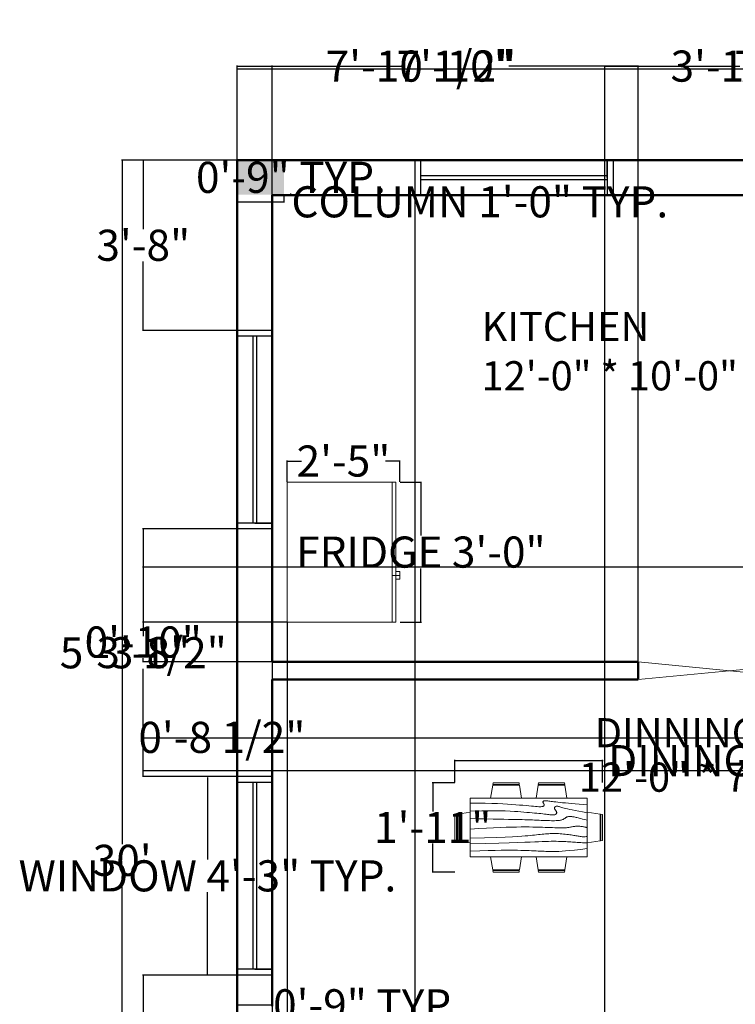
# Model space of a CAD drawing. Units: inches. Extents: x 9717 to 10218, y 17835 to 18358.
# Tile 2 of 4: x 9717 to 9901, y 18104 to 18358. Entities that reach past the tile are written whole.
import ezdxf

# ---------------------------------------------------------------- set-up
doc = ezdxf.new("R2010")
doc.units = ezdxf.units.IN
for name, color, linetype, lineweight in [('A-AREA-IDEN', 3, 'Continuous', 25), ('A-EQPM', 2, 'Continuous', 18), ('ARCHES', 5, 'Continuous', 18), ('COLUMN', 7, 'Continuous', 35), ('DIMENSIONS', 3, 'Continuous', 18), ('FURNITURES', 2, 'Continuous', 18), ('WALLS', 7, 'Continuous', 50), ('WINDOWS', 4, 'Continuous', 25)]:
    doc.layers.add(name, color=color, linetype=linetype, lineweight=lineweight)
doc.styles.get("Standard").update_dxf_attribs({"font": 'arial.ttf'})
doc.dimstyles.get("Standard").update_dxf_attribs({"dimtxt": 8, "dimasz": 0.18, "dimexe": 0.18, "dimexo": 0.0625, "dimgap": 0.09, "dimtad": 0, "dimtih": 1, "dimtoh": 1, "dimzin": 0, "dimdsep": 46, "dimlunit": 3, "dimtxsty": 'Standard', "dimcen": 0.09, "dimadec": 0, "dimazin": 0, "dimtfac": 1, "dimtofl": 0, "dimtmove": 0, "dimatfit": 3, "dimfxl": 1, "dimtolj": 1, "dimtzin": 0, "dimarcsym": 0})

# ---------------------------------------------------------------- blocks, each defined once
blk = doc.blocks.new('Dining Set - 36 x 72 in.')
for p, q in [((-22.2343, 26.00059), (-23.4847, 17.99762)), ((-22.2304, 26), (-5.7608, 26)), ((-22, 27.5), (-22.1562, 26.50042)), ((-5.8416, 26.5), (-22.1534, 26.5)), ((-22, 27.5), (-6, 27.5)), ((-5.8437, 26.49966), (-6, 27.5)), ((-4.5152, 17.99762), (-5.7655, 25.99926)), ((5.7657, 26.00059), (4.5153, 17.99762)), ((5.7696, 26), (22.2392, 26)), ((6, 27.5), (5.8438, 26.50042)), ((22.1584, 26.5), (5.8466, 26.5)), ((6, 27.5), (22, 27.5)), ((22.1563, 26.49966), (22, 27.5)), ((23.4848, 17.99762), (22.2345, 25.99926)), ((36, 18), (-36, 18)), ((-36, 18), (-36, -18)), ((36, -18), (36, 18)), ((-45.5, 8), (-44.5004, 8.15617)), ((-45.5, 8), (-45.5, -8)), ((-44.5, -8.15843), (-44.5, 8.15338)), ((-44.0006, 8.23428), (-35.9976, 9.48474)), ((-44, 8.23041), (-44, -8.23915)), ((44.0006, 8.23428), (35.9976, 9.48474)), ((44, 8.23041), (44, -8.23915)), ((44.5, -8.15843), (44.5, 8.15338)), ((45.5, 8), (44.5005, 8.15617)), ((45.5, 8), (45.5, -8)), ((-44.4997, -8.15631), (-45.5, -8)), ((-35.9976, -9.48476), (-43.9993, -8.2345)), ((35.9976, -9.48476), (43.9993, -8.2345)), ((44.4997, -8.15631), (45.5, -8)), ((-36, -18), (36, -18)), ((-22.2343, -26.0006), (-23.4847, -17.99762)), ((-4.5152, -17.99762), (-5.7655, -25.99928)), ((5.7657, -26.0006), (4.5153, -17.99762)), ((23.4848, -17.99762), (22.2345, -25.99928)), ((-22.2304, -26), (-5.7608, -26)), ((-22, -27.5), (-22.1562, -26.50044)), ((-5.8416, -26.5), (-22.1534, -26.5)), ((-22, -27.5), (-6, -27.5)), ((-5.8437, -26.49967), (-6, -27.5)), ((5.7696, -26), (22.2392, -26)), ((6, -27.5), (5.8438, -26.50044)), ((22.1584, -26.5), (5.8466, -26.5)), ((6, -27.5), (22, -27.5)), ((22.1563, -26.49967), (22, -27.5))]:
    blk.add_line(p, q)
for points in [[(-36, 15), (-31.1772, 14.97754), (-26.8079, 14.91406), (-22.8538, 14.81543), (-19.276, 14.6875), (-16.0362, 14.53613), (-13.0957, 14.36718), (-10.4159, 14.18652), (-7.9583, 14), (-5.6904, 13.81315), (-3.6035, 13.63021), (-1.6954, 13.45508), (0.0365, 13.29166), (1.5945, 13.14388), (2.9811, 13.01562), (4.1988, 12.9108), (5.25, 12.83333), (6.1393, 12.78613), (6.8802, 12.76823), (7.4883, 12.77767), (7.9792, 12.8125), (8.3685, 12.87077), (8.6719, 12.95052), (8.9049, 13.0498), (9.0833, 13.16666), (9.2205, 13.29899), (9.3216, 13.44401), (9.3895, 13.59879), (9.4271, 13.76041), (9.4373, 13.92594), (9.4232, 14.09245), (9.3875, 14.257), (9.3333, 14.41666), (9.2638, 14.56917), (9.1836, 14.71484), (9.0975, 14.85465), (9.0104, 14.98958), (8.9272, 15.1206), (8.8529, 15.2487), (8.7922, 15.37483), (8.75, 15.5), (8.7305, 15.62467), (8.7344, 15.74739), (8.7617, 15.86621), (8.8125, 15.97916), (8.8867, 16.08431), (8.9844, 16.17968), (9.1055, 16.26334), (9.25, 16.33333), (9.4189, 16.38802), (9.6172, 16.42708), (9.8506, 16.45052), (10.125, 16.45833), (10.4463, 16.45052), (10.8203, 16.42708), (11.2529, 16.38802), (11.75, 16.33333), (12.3184, 16.26318), (12.9694, 16.17838), (13.7151, 16.07991), (14.5677, 15.96875), (15.5395, 15.84586), (16.6426, 15.71224), (17.8893, 15.56884), (19.2917, 15.41666), (20.859, 15.25667), (22.5879, 15.08984), (24.4721, 14.91715), (26.5052, 14.73958), (28.6809, 14.5581), (30.9929, 14.3737), (33.4347, 14.18733), (36, 14)], [(-36, 10), (-28.9766, 10.14274), (-23.1725, 10.20442), (-18.4241, 10.19775), (-14.5677, 10.13541), (-11.4399, 10.03011), (-8.877, 9.89453), (-6.7154, 9.74137), (-4.7917, 9.58333), (-2.9698, 9.43082), (-1.2246, 9.28515), (0.4415, 9.14534), (2.026, 9.01041), (3.5266, 8.87939), (4.9408, 8.7513), (6.266, 8.62516), (7.5, 8.5), (8.6411, 8.37549), (9.6914, 8.2539), (10.6538, 8.13818), (11.5312, 8.03125), (12.3267, 7.93603), (13.043, 7.85547), (13.6831, 7.79248), (14.25, 7.75), (14.7471, 7.7303), (15.1797, 7.73307), (15.5537, 7.75732), (15.875, 7.80208), (16.1494, 7.86637), (16.3828, 7.94922), (16.5811, 8.04964), (16.75, 8.16666), (16.8944, 8.29915), (17.0143, 8.44531), (17.1089, 8.60319), (17.1771, 8.77083), (17.218, 8.94629), (17.2305, 9.1276), (17.2137, 9.31282), (17.1667, 9.5), (17.0895, 9.6875), (16.987, 9.875), (16.8649, 10.0625), (16.7292, 10.25), (16.5856, 10.4375), (16.4401, 10.625), (16.2985, 10.8125), (16.1667, 11), (16.05, 11.18733), (15.9518, 11.3737), (15.8752, 11.5581), (15.8229, 11.73958), (15.798, 11.91715), (15.8034, 12.08984), (15.842, 12.25667), (15.9167, 12.41666), (16.0295, 12.56836), (16.1784, 12.70833), (16.3605, 12.83268), (16.5729, 12.9375), (16.8127, 13.01888), (17.0768, 13.07291), (17.3625, 13.0957), (17.6667, 13.08333), (17.9894, 13.03312), (18.3418, 12.94726), (18.7382, 12.82918), (19.1927, 12.68229), (19.7195, 12.51001), (20.3327, 12.31575), (21.0465, 12.10294), (21.875, 11.875), (22.8357, 11.63354), (23.959, 11.37304), (25.2786, 11.08618), (26.8282, 10.76562), (28.6414, 10.40405), (30.752, 9.99414), (33.1936, 9.52856), (36, 9)], [(-36, 5.5), (-30.7157, 5.3348), (-26.069, 5.20963), (-21.9946, 5.11767), (-18.4271, 5.05208), (-15.3009, 5.00602), (-12.5508, 4.97265), (-10.1112, 4.94515), (-7.9167, 4.91666), (-5.909, 4.88167), (-4.0586, 4.83984), (-2.3429, 4.79215), (-0.7396, 4.73958), (0.7739, 4.6831), (2.22, 4.6237), (3.6213, 4.56233), (5, 4.5), (6.373, 4.43782), (7.7344, 4.3776), (9.0723, 4.32129), (10.375, 4.27083), (11.6309, 4.22819), (12.8281, 4.19531), (13.9551, 4.17415), (15, 4.16666), (15.954, 4.17448), (16.819, 4.19791), (17.6001, 4.23698), (18.3021, 4.29166), (18.9299, 4.36198), (19.4883, 4.44791), (19.9823, 4.54948), (20.4167, 4.66666), (20.7969, 4.79899), (21.1302, 4.94401), (21.4245, 5.09879), (21.6875, 5.26041), (21.9271, 5.42594), (22.1511, 5.59245), (22.3672, 5.757), (22.5834, 5.91666), (22.8065, 6.06868), (23.0404, 6.21093), (23.2879, 6.34147), (23.5521, 6.45833), (23.8358, 6.55957), (24.142, 6.64323), (24.4735, 6.70735), (24.8334, 6.75), (25.2235, 6.76969), (25.642, 6.76692), (26.0858, 6.74267), (26.5521, 6.69791), (27.0379, 6.63362), (27.5404, 6.55078), (28.0565, 6.45036), (28.5834, 6.33333), (29.1242, 6.19987), (29.7071, 6.04687), (30.3661, 5.87044), (31.1354, 5.66666), (32.0493, 5.43164), (33.142, 5.16146), (34.4475, 4.85221), (36, 4.5)], [(-36, -1), (-30.7915, -0.6591), (-26.0195, -0.38216), (-21.6519, -0.16284), (-17.6563, 0.00521), (-14.0005, 0.12833), (-10.6523, 0.21289), (-7.5796, 0.26522), (-4.75, 0.29166), (-2.134, 0.29793), (0.2878, 0.28711), (2.5317, 0.26163), (4.6146, 0.22396), (6.5529, 0.17651), (8.3633, 0.12174), (10.0623, 0.06209), (11.6667, 0), (13.1899, -0.06201), (14.6341, -0.1211), (15.9982, -0.17432), (17.2813, -0.21875), (18.4823, -0.25147), (19.6003, -0.26953), (20.6343, -0.27002), (21.5834, -0.25), (22.4481, -0.20768), (23.2357, -0.14584), (23.9549, -0.06836), (24.6146, 0.02083), (25.2235, 0.11784), (25.7904, 0.21875), (26.3241, 0.31966), (26.8334, 0.41666), (27.3265, 0.50618), (27.8099, 0.58593), (28.2894, 0.65397), (28.7709, 0.70833), (29.2601, 0.74707), (29.763, 0.76823), (30.2855, 0.76985), (30.8334, 0.75), (31.4088, 0.70784), (31.9994, 0.64713), (32.589, 0.57275), (33.1615, 0.48958), (33.7008, 0.4025), (34.1908, 0.3164), (34.6153, 0.23616), (34.9584, 0.16666), (35.2099, 0.11165), (35.3848, 0.07031), (35.504, 0.04069), (35.5886, 0.02083), (35.6594, 0.00879), (35.7377, 0.0026), (35.8442, 0.00032), (36, 0)], [(-36, -6.5), (-27.1843, -6.31267), (-20.084, -6.1263), (-14.469, -5.9419), (-10.1094, -5.76042), (-6.7752, -5.58285), (-4.2363, -5.41016), (-2.2629, -5.24333), (-0.625, -5.08334), (0.8708, -4.93099), (2.2715, -4.78646), (3.5872, -4.64974), (4.8281, -4.52084), (6.0046, -4.39974), (7.127, -4.28646), (8.2053, -4.18099), (9.25, -4.08334), (10.2705, -3.99382), (11.2734, -3.91407), (12.2647, -3.84603), (13.25, -3.79167), (14.2354, -3.75293), (15.2266, -3.73177), (16.2295, -3.73015), (17.25, -3.75), (18.2912, -3.79248), (19.3451, -3.85547), (20.4009, -3.93604), (21.4479, -4.03125), (22.4754, -4.13819), (23.4727, -4.25391), (24.4289, -4.37549), (25.3334, -4.5), (26.1785, -4.62492), (26.9694, -4.74935), (27.7145, -4.87281), (28.4219, -4.99479), (29.1, -5.11483), (29.7572, -5.23242), (30.4016, -5.34709), (31.0417, -5.45834), (31.6837, -5.56437), (32.3262, -5.65821), (32.9658, -5.73153), (33.599, -5.77604), (34.2224, -5.78345), (34.8327, -5.74545), (35.4264, -5.65373), (36, -5.5)], [(-36, -10), (-26.4022, -9.81299), (-18.4675, -9.62891), (-11.9839, -9.45069), (-6.7396, -9.28125), (-2.5226, -9.12354), (0.8789, -8.98047), (3.6769, -8.85498), (6.0833, -8.75), (8.2767, -8.66765), (10.3021, -8.60677), (12.1712, -8.56543), (13.8958, -8.54167), (15.4876, -8.53353), (16.9583, -8.53907), (18.3197, -8.55632), (19.5834, -8.58334), (20.7616, -8.61841), (21.8685, -8.66081), (22.9188, -8.71004), (23.9271, -8.76563), (24.9081, -8.82707), (25.8763, -8.89388), (26.8465, -8.96558), (27.8334, -9.04167), (28.8474, -9.12118), (29.8828, -9.20117), (30.93, -9.27824), (31.9792, -9.34896), (33.0205, -9.40991), (34.0443, -9.45768), (35.0407, -9.48885), (36, -9.5)], [(-36, -14.5), (-30.0881, -14.33513), (-25.0332, -14.21224), (-20.7312, -14.12647), (-17.0781, -14.07292), (-13.97, -14.04671), (-11.3027, -14.04297), (-8.9724, -14.05681), (-6.875, -14.08334), (-4.9224, -14.11833), (-3.0905, -14.16016), (-1.3709, -14.20785), (0.2448, -14.26042), (1.7647, -14.3169), (3.1973, -14.3763), (4.5507, -14.43767), (5.8333, -14.5), (7.0554, -14.5621), (8.235, -14.62175), (9.3922, -14.67652), (10.5469, -14.72396), (11.7192, -14.76164), (12.929, -14.78711), (14.1965, -14.79794), (15.5417, -14.79167), (16.9933, -14.76424), (18.6152, -14.70508), (20.4804, -14.60197), (22.6615, -14.44271), (25.2312, -14.21509), (28.2624, -13.9069), (31.8277, -13.50594), (36, -13)]]:
    blk.add_lwpolyline(points)
blk = doc.blocks.new('Refrigerator-2 door - 36 in top')
for p, q in [((0, -26.999999), (36, -26.999999)), ((12, -26.999999), (12, -28.999999)), ((11, -27.999999), (11, -28.999999)), ((11, -28.999999), (13, -28.999999)), ((13, -28.999999), (13, -27.999999))]:
    blk.add_line(p, q)
blk.add_lwpolyline([(0, -27.999999), (0, 0), (36, 0), (36, -27.999999)], close=True)
blk = doc.blocks.new('*D8')
at = {"layer": 'Defpoints', "color": 0, "transparency": 16777216}
for p in [(10150.76, 18344.92), (9772.76, 18321.49), (10150.76, 18321.49)]:
    blk.add_point(p, dxfattribs=at)
at = {"layer": 'DIMENSIONS', "color": 0, "lineweight": -2, "transparency": 16777216}
for p, q in [((9772.76, 18321.55), (9772.76, 18345.1)), ((9772.94, 18344.92), (9940.16, 18344.92)), ((10150.58, 18344.92), (9983.36, 18344.92)), ((10150.76, 18321.55), (10150.76, 18345.1))]:
    blk.add_line(p, q, dxfattribs=at)
at = {"layer": 'DIMENSIONS', "color": 0, "transparency": 16777216}
for points in [[(9772.94, 18344.95), (9772.94, 18344.89), (9772.76, 18344.92)], [(10150.58, 18344.95), (10150.58, 18344.89), (10150.76, 18344.92)]]:
    blk.add_solid(points, dxfattribs=at)
at = {"layer": 'DIMENSIONS', "color": 0, "transparency": 16777216, "insert": (9961.76, 18344.92), "char_height": 8, "attachment_point": 5}
blk.add_mtext('\\A1;31\'-6.00"', dxfattribs=at)
blk = doc.blocks.new('*D9')
at = {"layer": 'Defpoints', "color": 0, "transparency": 16777216}
for p in [(9772.76, 18321.49), (9743.19, 17961.49), (9772.76, 17961.49)]:
    blk.add_point(p, dxfattribs=at)
at = {"layer": 'DIMENSIONS', "color": 0, "lineweight": -2, "transparency": 16777216}
for p, q in [((9772.7, 18321.49), (9743.01, 18321.49)), ((9743.19, 18321.31), (9743.19, 18145.67)), ((9743.19, 17961.67), (9743.19, 18137.31)), ((9772.7, 17961.49), (9743.01, 17961.49))]:
    blk.add_line(p, q, dxfattribs=at)
at = {"layer": 'DIMENSIONS', "color": 0, "transparency": 16777216}
for points in [[(9743.16, 18321.31), (9743.22, 18321.31), (9743.19, 18321.49)], [(9743.16, 17961.67), (9743.22, 17961.67), (9743.19, 17961.49)]]:
    blk.add_solid(points, dxfattribs=at)
at = {"layer": 'DIMENSIONS', "color": 0, "transparency": 16777216, "insert": (9743.19, 18141.49), "char_height": 8, "attachment_point": 5}
blk.add_mtext("\\A1;30'", dxfattribs=at)
blk = doc.blocks.new('WIN-48IN')
for p, q in [((0.5, 9), (0, 9)), ((0, 9), (0, 0)), ((1, 9), (0.5, 9)), ((1.5, 9), (1, 9)), ((1.5, 9), (1.5, 0)), ((49.5, 4.5), (49.5, 9)), ((49.5, 9), (49.5, 0)), ((49.5, 9), (51, 9)), ((51, 9), (51, 0)), ((1.5, 5), (49.5, 5)), ((1.5, 4), (49.5, 4)), ((0, 0), (1.5, 0)), ((51, 0), (49.5, 0))]:
    blk.add_line(p, q)
blk = doc.blocks.new('COL-12X9IN')
h = blk.add_hatch(color=256)
h.dxf.hatch_style = 1
h.paths.add_polyline_path([(12, 0), (12, 9), (0, 9), (0, 0)])
blk = doc.blocks.new('*D14')
at = {"layer": 'Defpoints', "color": 0, "transparency": 16777216}
for p in [(9772.78, 18312.56), (9784.78, 18312.56), (9784.78, 18310.76)]:
    blk.add_point(p, dxfattribs=at)
at = {"layer": 'DIMENSIONS', "color": 0, "lineweight": -2, "transparency": 16777216}
for p, q in [((9772.78, 18312.5), (9772.78, 18310.58)), ((9772.96, 18310.76), (9784.6, 18310.76)), ((9784.78, 18312.5), (9784.78, 18310.58)), ((9784.78, 18310.76), (9784.96, 18310.76))]:
    blk.add_line(p, q, dxfattribs=at)
at = {"layer": 'DIMENSIONS', "color": 0, "transparency": 16777216}
for points in [[(9772.96, 18310.79), (9772.96, 18310.73), (9772.78, 18310.76)], [(9784.6, 18310.79), (9784.6, 18310.73), (9784.78, 18310.76)]]:
    blk.add_solid(points, dxfattribs=at)
at = {"layer": 'DIMENSIONS', "color": 0, "transparency": 16777216, "insert": (9835.15, 18310.76), "char_height": 8, "attachment_point": 5}
blk.add_mtext('\\A1;COLUMN 1\'-0" TYP.', dxfattribs=at)
blk = doc.blocks.new('*D15')
at = {"layer": 'Defpoints', "color": 0, "transparency": 16777216}
for p in [(9784.78, 18321.56), (9786.58, 18321.56), (9784.78, 18312.56)]:
    blk.add_point(p, dxfattribs=at)
at = {"layer": 'DIMENSIONS', "color": 0, "lineweight": -2, "transparency": 16777216}
for p, q in [((9784.84, 18321.56), (9786.76, 18321.56)), ((9786.58, 18321.38), (9786.58, 18321.23)), ((9786.58, 18312.74), (9786.58, 18312.88)), ((9784.84, 18312.56), (9786.76, 18312.56))]:
    blk.add_line(p, q, dxfattribs=at)
at = {"layer": 'DIMENSIONS', "color": 0, "transparency": 16777216}
for points in [[(9786.55, 18321.38), (9786.61, 18321.38), (9786.58, 18321.56)], [(9786.55, 18312.74), (9786.61, 18312.74), (9786.58, 18312.56)]]:
    blk.add_solid(points, dxfattribs=at)
at = {"layer": 'DIMENSIONS', "color": 0, "transparency": 16777216, "insert": (9786.58, 18317.06), "char_height": 8, "attachment_point": 5}
blk.add_mtext('\\A1;0\'-9" TYP.', dxfattribs=at)
blk = doc.blocks.new('*D16')
at = {"layer": 'Defpoints', "color": 0, "transparency": 16777216}
for p in [(9772.76, 18163.01), (9765.11, 18112.01), (9772.76, 18112.01)]:
    blk.add_point(p, dxfattribs=at)
at = {"layer": 'DIMENSIONS', "color": 0, "lineweight": -2, "transparency": 16777216}
for p, q in [((9772.7, 18163.01), (9764.93, 18163.01)), ((9765.11, 18162.83), (9765.11, 18141.74)), ((9765.11, 18112.19), (9765.11, 18133.28)), ((9772.7, 18112.01), (9764.93, 18112.01))]:
    blk.add_line(p, q, dxfattribs=at)
at = {"layer": 'DIMENSIONS', "color": 0, "transparency": 16777216}
for points in [[(9765.08, 18162.83), (9765.14, 18162.83), (9765.11, 18163.01)], [(9765.08, 18112.19), (9765.14, 18112.19), (9765.11, 18112.01)]]:
    blk.add_solid(points, dxfattribs=at)
at = {"layer": 'DIMENSIONS', "color": 0, "transparency": 16777216, "insert": (9765.11, 18137.51), "char_height": 8, "attachment_point": 5}
blk.add_mtext('\\A1;WINDOW 4\'-3" TYP.', dxfattribs=at)
blk = doc.blocks.new('*D17')
at = {"layer": 'Defpoints', "color": 0, "transparency": 16777216}
for p in [(9772.76, 18112.01), (9781.76, 18112.01), (9781.76, 18104.36)]:
    blk.add_point(p, dxfattribs=at)
at = {"layer": 'DIMENSIONS', "color": 0, "lineweight": -2, "transparency": 16777216}
for p, q in [((9772.76, 18111.95), (9772.76, 18104.18)), ((9781.76, 18111.95), (9781.76, 18104.18)), ((9772.94, 18104.36), (9781.58, 18104.36)), ((9781.76, 18104.36), (9781.94, 18104.36))]:
    blk.add_line(p, q, dxfattribs=at)
at = {"layer": 'DIMENSIONS', "color": 0, "transparency": 16777216}
for points in [[(9772.94, 18104.39), (9772.94, 18104.33), (9772.76, 18104.36)], [(9781.58, 18104.39), (9781.58, 18104.33), (9781.76, 18104.36)]]:
    blk.add_solid(points, dxfattribs=at)
at = {"layer": 'DIMENSIONS', "color": 0, "transparency": 16777216, "insert": (9806.41, 18104.36), "char_height": 8, "attachment_point": 5}
blk.add_mtext('\\A1;0\'-9" TYP.', dxfattribs=at)
blk = doc.blocks.new('*D28')
at = {"layer": 'Defpoints', "color": 0, "transparency": 16777216}
for p in [(9866.73, 18167.12), (9828.75, 18161.43), (9866.73, 18161.43)]:
    blk.add_point(p, dxfattribs=at)
at = {"layer": 'DIMENSIONS', "color": 0, "lineweight": -2, "transparency": 16777216}
for p, q in [((9828.75, 18161.49), (9828.75, 18167.3)), ((9828.93, 18167.12), (9866.55, 18167.12)), ((9866.73, 18161.49), (9866.73, 18167.3)), ((9866.73, 18167.12), (9866.91, 18167.12))]:
    blk.add_line(p, q, dxfattribs=at)
at = {"layer": 'DIMENSIONS', "color": 0, "transparency": 16777216}
for points in [[(9828.93, 18167.15), (9828.93, 18167.09), (9828.75, 18167.12)], [(9866.55, 18167.15), (9866.55, 18167.09), (9866.73, 18167.12)]]:
    blk.add_solid(points, dxfattribs=at)
at = {"layer": 'DIMENSIONS', "color": 0, "transparency": 16777216, "insert": (9910.97, 18167.12), "char_height": 8, "attachment_point": 5}
blk.add_mtext('\\A1;DINING SET 3\'-2"', dxfattribs=at)
blk = doc.blocks.new('*D29')
at = {"layer": 'Defpoints', "color": 0, "transparency": 16777216}
for p in [(9823.05, 18161.43), (9828.75, 18161.43), (9828.75, 18138.47)]:
    blk.add_point(p, dxfattribs=at)
at = {"layer": 'DIMENSIONS', "color": 0, "lineweight": -2, "transparency": 16777216}
for p, q in [((9828.69, 18161.43), (9822.87, 18161.43)), ((9823.05, 18161.25), (9823.05, 18154.05)), ((9823.05, 18138.65), (9823.05, 18145.84)), ((9828.69, 18138.47), (9822.87, 18138.47))]:
    blk.add_line(p, q, dxfattribs=at)
at = {"layer": 'DIMENSIONS', "color": 0, "transparency": 16777216}
for points in [[(9823.02, 18161.25), (9823.08, 18161.25), (9823.05, 18161.43)], [(9823.02, 18138.65), (9823.08, 18138.65), (9823.05, 18138.47)]]:
    blk.add_solid(points, dxfattribs=at)
at = {"layer": 'DIMENSIONS', "color": 0, "transparency": 16777216, "insert": (9823.05, 18149.95), "char_height": 8, "attachment_point": 5}
blk.add_mtext('\\A1;1\'-11"', dxfattribs=at)
blk = doc.blocks.new('*D30')
at = {"layer": 'Defpoints', "color": 0, "transparency": 16777216}
for p in [(9814.6, 18238.73), (9820, 18238.73), (9814.6, 18202.73)]:
    blk.add_point(p, dxfattribs=at)
at = {"layer": 'DIMENSIONS', "color": 0, "lineweight": -2, "transparency": 16777216}
for p, q in [((9814.66, 18238.73), (9820.18, 18238.73)), ((9820, 18238.55), (9820, 18224.96)), ((9820, 18202.91), (9820, 18216.51)), ((9814.66, 18202.73), (9820.18, 18202.73))]:
    blk.add_line(p, q, dxfattribs=at)
at = {"layer": 'DIMENSIONS', "color": 0, "transparency": 16777216}
for points in [[(9819.97, 18238.55), (9820.03, 18238.55), (9820, 18238.73)], [(9819.97, 18202.91), (9820.03, 18202.91), (9820, 18202.73)]]:
    blk.add_solid(points, dxfattribs=at)
at = {"layer": 'DIMENSIONS', "color": 0, "transparency": 16777216, "insert": (9820, 18220.73), "char_height": 8, "attachment_point": 5}
blk.add_mtext('\\A1;FRIDGE 3\'-0"', dxfattribs=at)
blk = doc.blocks.new('*D31')
at = {"layer": 'Defpoints', "color": 0, "transparency": 16777216}
for p in [(9785.6, 18244.13), (9785.6, 18238.73), (9814.6, 18238.73)]:
    blk.add_point(p, dxfattribs=at)
at = {"layer": 'DIMENSIONS', "color": 0, "lineweight": -2, "transparency": 16777216}
for p, q in [((9785.6, 18238.8), (9785.6, 18244.31)), ((9785.78, 18244.13), (9789.31, 18244.13)), ((9814.42, 18244.13), (9810.89, 18244.13)), ((9814.6, 18238.8), (9814.6, 18244.31))]:
    blk.add_line(p, q, dxfattribs=at)
at = {"layer": 'DIMENSIONS', "color": 0, "transparency": 16777216}
for points in [[(9785.78, 18244.16), (9785.78, 18244.1), (9785.6, 18244.13)], [(9814.42, 18244.16), (9814.42, 18244.1), (9814.6, 18244.13)]]:
    blk.add_solid(points, dxfattribs=at)
at = {"layer": 'DIMENSIONS', "color": 0, "transparency": 16777216, "insert": (9800.1, 18244.13), "char_height": 8, "attachment_point": 5}
blk.add_mtext('\\A1;2\'-5"', dxfattribs=at)
blk = doc.blocks.new('*D32')
at = {"layer": 'Defpoints', "color": 0, "transparency": 16777216}
for p in [(9867.28, 18345.64), (9867.28, 17970.49), (9772.76, 17961.49)]:
    blk.add_point(p, dxfattribs=at)
at = {"layer": 'DIMENSIONS', "color": 0, "lineweight": -2, "transparency": 16777216}
for p, q in [((9772.76, 17961.55), (9772.76, 18345.82)), ((9867.28, 17970.55), (9867.28, 18345.82)), ((9772.94, 18345.64), (9796.9, 18345.64)), ((9867.1, 18345.64), (9843.14, 18345.64))]:
    blk.add_line(p, q, dxfattribs=at)
at = {"layer": 'DIMENSIONS', "color": 0, "transparency": 16777216}
for points in [[(9772.94, 18345.67), (9772.94, 18345.61), (9772.76, 18345.64)], [(9867.1, 18345.67), (9867.1, 18345.61), (9867.28, 18345.64)]]:
    blk.add_solid(points, dxfattribs=at)
at = {"layer": 'DIMENSIONS', "color": 0, "transparency": 16777216, "insert": (9820.02, 18345.64), "char_height": 8, "attachment_point": 5}
blk.add_mtext('\\A1;7\'-10 1/2"', dxfattribs=at)
blk = doc.blocks.new('*D33')
at = {"layer": 'Defpoints', "color": 0, "transparency": 16777216}
for p in [(9958.06, 18345.64), (9867.28, 17970.49), (9958.06, 17970.49)]:
    blk.add_point(p, dxfattribs=at)
at = {"layer": 'DIMENSIONS', "color": 0, "lineweight": -2, "transparency": 16777216}
for p, q in [((9867.28, 17970.55), (9867.28, 18345.82)), ((9958.06, 17970.55), (9958.06, 18345.82)), ((9867.46, 18345.64), (9901.98, 18345.64)), ((9957.88, 18345.64), (9923.36, 18345.64))]:
    blk.add_line(p, q, dxfattribs=at)
at = {"layer": 'DIMENSIONS', "color": 0, "transparency": 16777216}
for points in [[(9867.46, 18345.67), (9867.46, 18345.61), (9867.28, 18345.64)], [(9957.88, 18345.67), (9957.88, 18345.61), (9958.06, 18345.64)]]:
    blk.add_solid(points, dxfattribs=at)
at = {"layer": 'DIMENSIONS', "color": 0, "transparency": 16777216, "insert": (9912.67, 18345.64), "char_height": 8, "attachment_point": 5}
blk.add_mtext('\\A1;7\'-7"', dxfattribs=at)
blk = doc.blocks.new('*D40')
at = {"layer": 'Defpoints', "color": 0, "transparency": 16777216}
for p in [(9781.76, 18312.49), (9818.43, 18312.49), (9818.43, 17847.34)]:
    blk.add_point(p, dxfattribs=at)
at = {"layer": 'DIMENSIONS', "color": 0, "lineweight": -2, "transparency": 16777216}
for p, q in [((9781.76, 18312.43), (9781.76, 17847.16)), ((9818.43, 18312.43), (9818.43, 17847.16)), ((9781.94, 17847.34), (9818.25, 17847.34)), ((9818.43, 17847.34), (9818.61, 17847.34))]:
    blk.add_line(p, q, dxfattribs=at)
at = {"layer": 'DIMENSIONS', "color": 0, "transparency": 16777216}
for points in [[(9781.94, 17847.37), (9781.94, 17847.31), (9781.76, 17847.34)], [(9818.25, 17847.37), (9818.25, 17847.31), (9818.43, 17847.34)]]:
    blk.add_solid(points, dxfattribs=at)
at = {"layer": 'DIMENSIONS', "color": 0, "transparency": 16777216, "insert": (9838.65, 17847.34), "char_height": 8, "attachment_point": 5}
blk.add_mtext('\\A1;3\'-0 1/2"', dxfattribs=at)
blk = doc.blocks.new('*D42')
at = {"layer": 'Defpoints', "color": 0, "transparency": 16777216}
for p in [(9772.76, 18321.49), (9748.61, 18277.7), (9772.76, 18277.7)]:
    blk.add_point(p, dxfattribs=at)
at = {"layer": 'DIMENSIONS', "color": 0, "lineweight": -2, "transparency": 16777216}
for p, q in [((9772.7, 18321.49), (9748.43, 18321.49)), ((9748.61, 18321.31), (9748.61, 18303.77)), ((9748.61, 18277.88), (9748.61, 18295.42)), ((9772.7, 18277.7), (9748.43, 18277.7))]:
    blk.add_line(p, q, dxfattribs=at)
at = {"layer": 'DIMENSIONS', "color": 0, "transparency": 16777216}
for points in [[(9748.58, 18321.31), (9748.64, 18321.31), (9748.61, 18321.49)], [(9748.58, 18277.88), (9748.64, 18277.88), (9748.61, 18277.7)]]:
    blk.add_solid(points, dxfattribs=at)
at = {"layer": 'DIMENSIONS', "color": 0, "transparency": 16777216, "insert": (9748.61, 18299.59), "char_height": 8, "attachment_point": 5}
blk.add_mtext('\\A1;3\'-8"', dxfattribs=at)
blk = doc.blocks.new('*D43')
at = {"layer": 'Defpoints', "color": 0, "transparency": 16777216}
for p in [(9748.61, 18226.7), (9772.76, 18226.7), (9772.76, 18163.01)]:
    blk.add_point(p, dxfattribs=at)
at = {"layer": 'DIMENSIONS', "color": 0, "lineweight": -2, "transparency": 16777216}
for p, q in [((9772.7, 18226.7), (9748.43, 18226.7)), ((9748.61, 18226.52), (9748.61, 18199.08)), ((9748.61, 18163.19), (9748.61, 18190.62)), ((9772.7, 18163.01), (9748.43, 18163.01))]:
    blk.add_line(p, q, dxfattribs=at)
at = {"layer": 'DIMENSIONS', "color": 0, "transparency": 16777216}
for points in [[(9748.58, 18226.52), (9748.64, 18226.52), (9748.61, 18226.7)], [(9748.58, 18163.19), (9748.64, 18163.19), (9748.61, 18163.01)]]:
    blk.add_solid(points, dxfattribs=at)
at = {"layer": 'DIMENSIONS', "color": 0, "transparency": 16777216, "insert": (9748.61, 18194.85), "char_height": 8, "attachment_point": 5}
blk.add_mtext('\\A1;5\'-3 1/2"', dxfattribs=at)
blk = doc.blocks.new('*D44')
at = {"layer": 'Defpoints', "color": 0, "transparency": 16777216}
for p in [(9748.61, 18112.01), (9772.76, 18112.01), (9772.76, 18056.11)]:
    blk.add_point(p, dxfattribs=at)
at = {"layer": 'DIMENSIONS', "color": 0, "lineweight": -2, "transparency": 16777216}
for p, q in [((9772.7, 18112.01), (9748.43, 18112.01)), ((9748.61, 18111.83), (9748.61, 18088.23)), ((9748.61, 18056.29), (9748.61, 18079.88)), ((9772.7, 18056.11), (9748.43, 18056.11))]:
    blk.add_line(p, q, dxfattribs=at)
at = {"layer": 'DIMENSIONS', "color": 0, "transparency": 16777216}
for points in [[(9748.58, 18111.83), (9748.64, 18111.83), (9748.61, 18112.01)], [(9748.58, 18056.29), (9748.64, 18056.29), (9748.61, 18056.11)]]:
    blk.add_solid(points, dxfattribs=at)
at = {"layer": 'DIMENSIONS', "color": 0, "transparency": 16777216, "insert": (9748.61, 18084.06), "char_height": 8, "attachment_point": 5}
blk.add_mtext('\\A1;4\'-8"', dxfattribs=at)
blk = doc.blocks.new('*D48')
at = {"layer": 'Defpoints', "color": 0, "transparency": 16777216}
for p in [(9875.9, 18345.64), (9781.76, 18192.49), (9875.9, 18192.49)]:
    blk.add_point(p, dxfattribs=at)
at = {"layer": 'DIMENSIONS', "color": 0, "lineweight": -2, "transparency": 16777216}
for p, q in [((9781.76, 18192.55), (9781.76, 18345.82)), ((9875.9, 18192.55), (9875.9, 18345.82)), ((9781.94, 18345.64), (9815.03, 18345.64)), ((9875.72, 18345.64), (9842.63, 18345.64))]:
    blk.add_line(p, q, dxfattribs=at)
at = {"layer": 'DIMENSIONS', "color": 0, "transparency": 16777216}
for points in [[(9781.94, 18345.67), (9781.94, 18345.61), (9781.76, 18345.64)], [(9875.72, 18345.67), (9875.72, 18345.61), (9875.9, 18345.64)]]:
    blk.add_solid(points, dxfattribs=at)
at = {"layer": 'DIMENSIONS', "color": 0, "transparency": 16777216, "insert": (9828.83, 18345.64), "char_height": 8, "attachment_point": 5}
blk.add_mtext('\\A1;7\'-10"', dxfattribs=at)
blk = doc.blocks.new('*D49')
at = {"layer": 'Defpoints', "color": 0, "transparency": 16777216}
for p in [(9922.68, 18345.64), (9875.9, 18192.49), (9922.68, 18192.49)]:
    blk.add_point(p, dxfattribs=at)
at = {"layer": 'DIMENSIONS', "color": 0, "lineweight": -2, "transparency": 16777216}
for p, q in [((9875.9, 18192.55), (9875.9, 18345.82)), ((9922.68, 18192.55), (9922.68, 18345.82)), ((9876.08, 18345.64), (9885.46, 18345.64)), ((9922.5, 18345.64), (9913.12, 18345.64))]:
    blk.add_line(p, q, dxfattribs=at)
at = {"layer": 'DIMENSIONS', "color": 0, "transparency": 16777216}
for points in [[(9876.08, 18345.67), (9876.08, 18345.61), (9875.9, 18345.64)], [(9922.5, 18345.67), (9922.5, 18345.61), (9922.68, 18345.64)]]:
    blk.add_solid(points, dxfattribs=at)
at = {"layer": 'DIMENSIONS', "color": 0, "transparency": 16777216, "insert": (9899.29, 18345.64), "char_height": 8, "attachment_point": 5}
blk.add_mtext('\\A1;3\'-11"', dxfattribs=at)
blk = doc.blocks.new('*D52')
at = {"layer": 'Defpoints', "color": 0, "transparency": 16777216}
for p in [(9748.61, 18216.87), (9993.26, 18216.87), (9993.26, 18172.92)]:
    blk.add_point(p, dxfattribs=at)
at = {"layer": 'DIMENSIONS', "color": 0, "lineweight": -2, "transparency": 16777216}
for p, q in [((9993.2, 18216.87), (9748.43, 18216.87)), ((9748.61, 18216.69), (9748.61, 18199.08)), ((9748.61, 18173.1), (9748.61, 18190.72)), ((9993.2, 18172.92), (9748.43, 18172.92))]:
    blk.add_line(p, q, dxfattribs=at)
at = {"layer": 'DIMENSIONS', "color": 0, "transparency": 16777216}
for points in [[(9748.58, 18216.69), (9748.64, 18216.69), (9748.61, 18216.87)], [(9748.58, 18173.1), (9748.64, 18173.1), (9748.61, 18172.92)]]:
    blk.add_solid(points, dxfattribs=at)
at = {"layer": 'DIMENSIONS', "color": 0, "transparency": 16777216, "insert": (9748.61, 18194.9), "char_height": 8, "attachment_point": 5}
blk.add_mtext('\\A1;3\'-8"', dxfattribs=at)
blk = doc.blocks.new('*D61')
at = {"layer": 'Defpoints', "color": 0, "transparency": 16777216}
for p in [(9748.61, 18172.92), (9993.26, 18172.92), (9993.26, 18164.49)]:
    blk.add_point(p, dxfattribs=at)
at = {"layer": 'DIMENSIONS', "color": 0, "lineweight": -2, "transparency": 16777216}
for p, q in [((9993.2, 18172.92), (9748.43, 18172.92)), ((9748.61, 18172.92), (9748.61, 18173.1)), ((9748.61, 18173.1), (9748.79, 18173.1)), ((9748.61, 18164.67), (9748.61, 18172.74)), ((9993.2, 18164.49), (9748.43, 18164.49))]:
    blk.add_line(p, q, dxfattribs=at)
at = {"layer": 'DIMENSIONS', "color": 0, "transparency": 16777216}
for points in [[(9748.58, 18172.74), (9748.64, 18172.74), (9748.61, 18172.92)], [(9748.58, 18164.67), (9748.64, 18164.67), (9748.61, 18164.49)]]:
    blk.add_solid(points, dxfattribs=at)
at = {"layer": 'DIMENSIONS', "color": 0, "transparency": 16777216, "insert": (9768.83, 18173.1), "char_height": 8, "attachment_point": 5}
blk.add_mtext('\\A1;0\'-8 1/2"', dxfattribs=at)
blk = doc.blocks.new('*D62')
at = {"layer": 'Defpoints', "color": 0, "transparency": 16777216}
for p in [(9785.597893, 18202.734969), (9781.760349, 18192.491492), (9785.597893, 17847.341492)]:
    blk.add_point(p, dxfattribs=at)
at = {"layer": 'DIMENSIONS', "color": 0, "lineweight": -2, "transparency": 16777216}
for p, q in [((9785.597893, 18202.672469), (9785.597893, 17847.161492)), ((9781.760349, 18192.428992), (9781.760349, 17847.161492)), ((9781.940349, 17847.341492), (9785.417893, 17847.341492)), ((9785.597893, 17847.341492), (9785.777893, 17847.341492))]:
    blk.add_line(p, q, dxfattribs=at)
at = {"layer": 'DIMENSIONS', "color": 0, "transparency": 16777216}
for points in [[(9781.940349, 17847.371492), (9781.940349, 17847.311492), (9781.760349, 17847.341492)], [(9785.417893, 17847.371492), (9785.417893, 17847.311492), (9785.597893, 17847.341492)]]:
    blk.add_solid(points, dxfattribs=at)
at = {"layer": 'DIMENSIONS', "color": 0, "transparency": 16777216, "insert": (9796.500908, 17847.341492), "char_height": 8, "attachment_point": 5}
blk.add_mtext('\\A1;0\'-4"', dxfattribs=at)
blk = doc.blocks.new('*D63')
at = {"layer": 'Defpoints', "color": 0, "transparency": 16777216}
for p in [(9748.61, 18202.73), (9785.6, 18202.73), (9781.76, 18192.49)]:
    blk.add_point(p, dxfattribs=at)
at = {"layer": 'DIMENSIONS', "color": 0, "lineweight": -2, "transparency": 16777216}
for p, q in [((9785.54, 18202.73), (9748.43, 18202.73)), ((9748.61, 18202.55), (9748.61, 18201.79)), ((9781.7, 18192.49), (9748.43, 18192.49)), ((9748.61, 18192.67), (9748.61, 18193.44))]:
    blk.add_line(p, q, dxfattribs=at)
at = {"layer": 'DIMENSIONS', "color": 0, "transparency": 16777216}
for points in [[(9748.58, 18202.55), (9748.64, 18202.55), (9748.61, 18202.73)], [(9748.58, 18192.67), (9748.64, 18192.67), (9748.61, 18192.49)]]:
    blk.add_solid(points, dxfattribs=at)
at = {"layer": 'DIMENSIONS', "color": 0, "transparency": 16777216, "insert": (9748.61, 18197.61), "char_height": 8, "attachment_point": 5}
blk.add_mtext('\\A1;0\'-10"', dxfattribs=at)

msp = doc.modelspace()

# ---------------------------------------------------------------- linework, layer by layer
at = {"layer": 'ARCHES'}
for p, q in [((9875.896, 18192.491), (9875.896, 18187.991)), ((9875.896, 18192.491), (9922.682, 18187.991)), ((9922.682, 18192.491), (9875.896, 18187.991))]:
    msp.add_line(p, q, dxfattribs=at)
at = {"layer": 'WALLS'}
for p, q in [((9781.76, 18312.491), (9925.76, 18312.491)), ((9781.76, 18192.491), (9781.76, 18312.491)), ((9781.76, 18192.491), (9875.896, 18192.491)), ((9875.896, 18192.491), (9875.896, 18187.991)), ((9781.76, 18187.991), (9875.896, 18187.991)), ((9781.76, 18103.991), (9781.76, 18187.991))]:
    msp.add_line(p, q, dxfattribs=at)
msp.add_lwpolyline([(9867.276, 17961.491), (9772.76, 17961.491), (9772.76, 18321.491), (10150.76, 18321.491), (10150.76, 17961.491)], dxfattribs=at)

# ---------------------------------------------------------------- block references
at = {"layer": 'A-EQPM', "rotation": 90}
msp.add_blockref('Refrigerator-2 door - 36 in top', (9785.598, 18202.735), dxfattribs=at)
at = {"layer": 'COLUMN'}
msp.add_blockref('COL-12X9IN', (9772.775, 18312.559), dxfattribs=at)
at = {"layer": 'FURNITURES', "xscale": 0.4174010763984445, "yscale": 0.4174010763984445, "zscale": 0.4174010763984445}
msp.add_blockref('Dining Set - 36 x 72 in.', (9847.742, 18149.948), dxfattribs=at)
at = {"layer": 'WINDOWS'}
msp.add_blockref('WIN-48IN', (9818.425, 18312.491), dxfattribs=at)
for p, rotation in [((9772.76, 18277.695), 270.0000000000058), ((9772.76, 18163.01), 270.0000000000044)]:
    msp.add_blockref('WIN-48IN', p, dxfattribs=dict(at, rotation=rotation))

# ---------------------------------------------------------------- texts
at = {"layer": 'A-AREA-IDEN'}
for s, p in [('KITCHEN', (9835.61, 18274.951)), ('12\'-0" * 10\'-0"', (9835.61, 18262.295)), ('DINNING', (9864.707, 18170.542)), ('12\'-0" * 7\'-0"', (9860.657, 18159.128))]:
    msp.add_text(s, height=7.5, dxfattribs=at).set_placement(p)

# ---------------------------------------------------------------- dimensions: what is measured, and where the dimension line sits
at = {"layer": 'DIMENSIONS'}
for base, p1, p2, override, picture, middle in [((9867.276, 18345.641), (9772.76, 17961.491), (9867.276, 17970.491), {"dimdec": 1, "dimlfac": 1, "dimrnd": 0, "dimzin": 1, "dimdsep": 46, "dimlunit": 4, "dimfrac": 2}, '*D32', (9820.018, 18345.641)), ((9875.896, 18345.641), (9781.76, 18192.491), (9875.896, 18192.491), {"dimdec": 1, "dimlfac": 1, "dimrnd": 0, "dimzin": 1, "dimdsep": 46, "dimlunit": 4, "dimfrac": 2}, '*D48', (9828.828, 18345.641)), ((9958.06, 18345.641), (9867.276, 17970.491), (9958.06, 17970.491), {"dimdec": 1, "dimlfac": 1, "dimrnd": 0, "dimzin": 1, "dimdsep": 46, "dimlunit": 4, "dimfrac": 2}, '*D33', (9912.668, 18345.641)), ((9922.682, 18345.641), (9875.896, 18192.491), (9922.682, 18192.491), {"dimdec": 1, "dimlfac": 1, "dimrnd": 0, "dimzin": 1, "dimdsep": 46, "dimlunit": 4, "dimfrac": 2}, '*D49', (9899.289, 18345.641)), ((10150.76, 18344.922), (9772.76, 18321.491), (10150.76, 18321.491), {"dimclrd": 0, "dimclre": 0, "dimclrt": 0}, '*D8', (9961.76, 18344.922)), ((9818.425, 17847.341), (9781.76, 18312.491), (9818.425, 18312.491), {"dimdec": 1, "dimlfac": 1, "dimrnd": 0, "dimzin": 1, "dimdsep": 46, "dimlunit": 4, "dimfrac": 2}, '*D40', (9838.646, 17847.341)), ((9785.598, 17847.341), (9781.76, 18192.491), (9785.598, 18202.735), {"dimdec": 1, "dimlfac": 1, "dimrnd": 0, "dimzin": 1, "dimdsep": 46, "dimlunit": 4, "dimfrac": 2}, '*D62', (9796.501, 17847.341))]:
    dim = msp.add_linear_dim(base=base, p1=p1, p2=p2, dimstyle='Standard', override=override, dxfattribs=at)
    dim.commit()
    dim.dimension.update_dxf_attribs({"geometry": picture, "text_midpoint": middle})
for base, p1, p2, angle, text, picture, middle in [((9786.575, 18321.559), (9784.775, 18312.559), (9784.775, 18321.559), 90, '<> TYP.', '*D15', (9786.575, 18317.059)), ((9819.998, 18238.735), (9814.598, 18202.735), (9814.598, 18238.735), 90, 'FRIDGE <>', '*D30', (9819.998, 18220.735)), ((9765.11, 18112.01), (9772.76, 18163.01), (9772.76, 18112.01), 270, 'WINDOW <> TYP.', '*D16', (9765.11, 18137.51))]:
    dim = msp.add_linear_dim(base=base, p1=p1, p2=p2, angle=angle, text=text, dimstyle='Standard', override={"dimdec": 1, "dimlfac": 1, "dimrnd": 0, "dimzin": 1, "dimdsep": 46, "dimlunit": 4, "dimfrac": 2}, dxfattribs=at)
    dim.commit()
    dim.dimension.update_dxf_attribs({"geometry": picture, "text_midpoint": middle})
for base, p1, p2, text, picture, middle in [((9784.775, 18310.759), (9772.775, 18312.559), (9784.775, 18312.559), 'COLUMN <> TYP.', '*D14', (9835.149, 18310.759)), ((9866.734, 18167.124), (9828.75, 18161.426), (9866.734, 18161.426), 'DINING SET <>', '*D28', (9910.968, 18167.124)), ((9781.76, 18104.36), (9772.76, 18112.01), (9781.76, 18112.01), '<> TYP.', '*D17', (9806.412, 18104.36))]:
    dim = msp.add_linear_dim(base=base, p1=p1, p2=p2, text=text, dimstyle='Standard', override={"dimdec": 1, "dimlfac": 1, "dimrnd": 0, "dimzin": 1, "dimdsep": 46, "dimlunit": 4, "dimfrac": 2}, dxfattribs=at)
    dim.commit()
    dim.dimension.update_dxf_attribs({"geometry": picture, "text_midpoint": middle})
for base, p1, p2, angle, override, picture, middle in [((9743.192, 17961.491), (9772.76, 18321.491), (9772.76, 17961.491), 90, {"dimclrd": 0, "dimclre": 0, "dimclrt": 0}, '*D9', (9743.192, 18141.491)), ((9748.61, 18277.695), (9772.76, 18321.491), (9772.76, 18277.695), 90, {"dimdec": 1, "dimlfac": 1, "dimrnd": 0, "dimzin": 1, "dimdsep": 46, "dimlunit": 4, "dimfrac": 2}, '*D42', (9748.61, 18299.593)), ((9785.598, 18244.135), (9814.598, 18238.735), (9785.598, 18238.735), 180, {"dimdec": 1, "dimlfac": 1, "dimrnd": 0, "dimzin": 1, "dimdsep": 46, "dimlunit": 4, "dimfrac": 2}, '*D31', (9800.098, 18244.135)), ((9748.61, 18226.695), (9772.76, 18163.01), (9772.76, 18226.695), 90, {"dimdec": 1, "dimlfac": 1, "dimrnd": 0, "dimzin": 1, "dimdsep": 46, "dimlunit": 4, "dimfrac": 2}, '*D43', (9748.61, 18194.853)), ((9748.61, 18216.874), (9993.26, 18172.923), (9993.26, 18216.874), 90, {"dimdec": 1, "dimlfac": 1, "dimrnd": 0, "dimzin": 1, "dimdsep": 46, "dimlunit": 4, "dimfrac": 2}, '*D52', (9748.61, 18194.899)), ((9748.61, 18202.735), (9781.76, 18192.491), (9785.598, 18202.735), 90, {"dimdec": 1, "dimlfac": 1, "dimrnd": 0, "dimzin": 1, "dimdsep": 46, "dimlunit": 4, "dimfrac": 2}, '*D63', (9748.61, 18197.613)), ((9748.61, 18172.923), (9993.26, 18164.491), (9993.26, 18172.923), 90, {"dimdec": 1, "dimlfac": 1, "dimrnd": 0, "dimzin": 1, "dimdsep": 46, "dimlunit": 4, "dimfrac": 2}, '*D61', (9768.834, 18173.103)), ((9823.053, 18161.426), (9828.75, 18138.469), (9828.75, 18161.426), 90, {"dimdec": 1, "dimlfac": 1, "dimrnd": 0, "dimzin": 1, "dimdsep": 46, "dimlunit": 4, "dimfrac": 2}, '*D29', (9823.053, 18149.948)), ((9748.61, 18112.01), (9772.76, 18056.108), (9772.76, 18112.01), 90, {"dimdec": 1, "dimlfac": 1, "dimrnd": 0, "dimzin": 1, "dimdsep": 46, "dimlunit": 4, "dimfrac": 2}, '*D44', (9748.61, 18084.059))]:
    dim = msp.add_linear_dim(base=base, p1=p1, p2=p2, angle=angle, dimstyle='Standard', override=override, dxfattribs=at)
    dim.commit()
    dim.dimension.update_dxf_attribs({"geometry": picture, "text_midpoint": middle})

doc.saveas('drawing.dxf')
